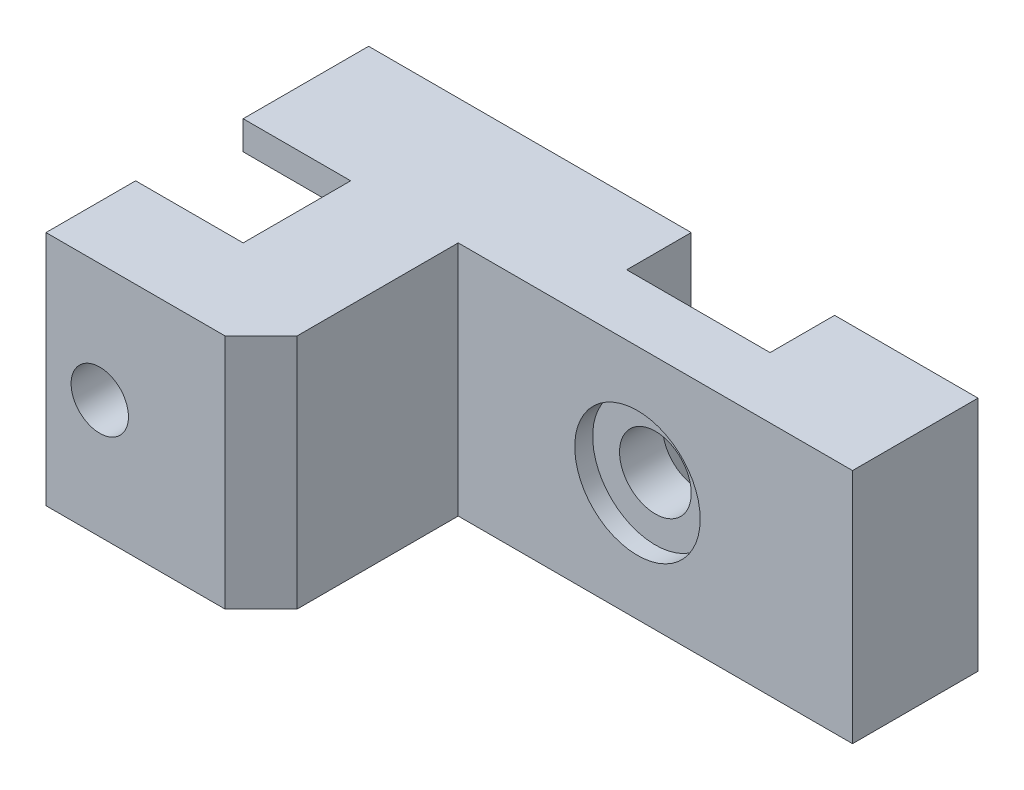
ISO-10303-21;
HEADER;
FILE_DESCRIPTION(('STEP AP214'),'2;1');
FILE_NAME('part.step','',(''),(''),'','','');
FILE_SCHEMA(('AUTOMOTIVE_DESIGN { 1 0 10303 214 1 1 1 1 }'));
ENDSEC;
DATA;
#1=APPLICATION_CONTEXT('core data for automotive mechanical design processes');
#2=APPLICATION_PROTOCOL_DEFINITION('international standard','automotive_design',2000,#1);
#3=PRODUCT_CONTEXT('',#1,'mechanical');
#4=PRODUCT('Part','Part','',(#3));
#5=PRODUCT_RELATED_PRODUCT_CATEGORY('part','',(#4));
#6=PRODUCT_DEFINITION_FORMATION('','',#4);
#7=PRODUCT_DEFINITION_CONTEXT('part definition',#1,'design');
#8=PRODUCT_DEFINITION('design','',#6,#7);
#9=PRODUCT_DEFINITION_SHAPE('','',#8);
#10=(LENGTH_UNIT() NAMED_UNIT(*) SI_UNIT(.MILLI.,.METRE.));
#11=(NAMED_UNIT(*) PLANE_ANGLE_UNIT() SI_UNIT($,.RADIAN.));
#12=(NAMED_UNIT(*) SI_UNIT($,.STERADIAN.) SOLID_ANGLE_UNIT());
#13=UNCERTAINTY_MEASURE_WITH_UNIT(LENGTH_MEASURE(1.E-05),#10,'distance_accuracy_value','');
#14=(GEOMETRIC_REPRESENTATION_CONTEXT(3) GLOBAL_UNCERTAINTY_ASSIGNED_CONTEXT((#13)) GLOBAL_UNIT_ASSIGNED_CONTEXT((#10,
#11,#12)) REPRESENTATION_CONTEXT('',''));
#15=CARTESIAN_POINT('',(0.,0.,0.));
#16=DIRECTION('',(0.,0.,1.));
#17=DIRECTION('',(1.,0.,0.));
#18=AXIS2_PLACEMENT_3D('',#15,#16,#17);
#19=CARTESIAN_POINT('',(0.,0.,35.));
#20=DIRECTION('',(0.,0.,1.));
#21=DIRECTION('',(1.,0.,0.));
#22=AXIS2_PLACEMENT_3D('',#19,#20,#21);
#23=PLANE('',#22);
#24=CARTESIAN_POINT('',(110.,33.,35.));
#25=DIRECTION('',(0.,0.,1.));
#26=DIRECTION('',(1.,0.,0.));
#27=AXIS2_PLACEMENT_3D('',#24,#25,#26);
#28=CIRCLE('',#27,17.5);
#29=CARTESIAN_POINT('',(127.5,33.,35.));
#30=VERTEX_POINT('',#29);
#31=EDGE_CURVE('E251',#30,#30,#28,.T.);
#32=ORIENTED_EDGE('',*,*,#31,.F.);
#33=EDGE_LOOP('',(#32));
#34=FACE_BOUND('',#33,.T.);
#35=DIRECTION('',(-1.,0.,0.));
#36=VECTOR('',#35,1.);
#37=CARTESIAN_POINT('',(170.,66.,35.));
#38=LINE('',#37,#36);
#39=CARTESIAN_POINT('',(170.,66.,35.));
#40=VERTEX_POINT('',#39);
#41=CARTESIAN_POINT('',(60.,66.,35.));
#42=VERTEX_POINT('',#41);
#43=EDGE_CURVE('E291',#40,#42,#38,.T.);
#44=ORIENTED_EDGE('',*,*,#43,.T.);
#45=DIRECTION('',(0.,-1.,0.));
#46=VECTOR('',#45,1.);
#47=CARTESIAN_POINT('',(60.,66.,35.));
#48=LINE('',#47,#46);
#49=CARTESIAN_POINT('',(60.,0.,35.));
#50=VERTEX_POINT('',#49);
#51=EDGE_CURVE('E230',#42,#50,#48,.T.);
#52=ORIENTED_EDGE('',*,*,#51,.T.);
#53=DIRECTION('',(1.,0.,0.));
#54=VECTOR('',#53,1.);
#55=CARTESIAN_POINT('',(0.,0.,35.));
#56=LINE('',#55,#54);
#57=CARTESIAN_POINT('',(170.,0.,35.));
#58=VERTEX_POINT('',#57);
#59=EDGE_CURVE('E288',#50,#58,#56,.T.);
#60=ORIENTED_EDGE('',*,*,#59,.T.);
#61=DIRECTION('',(0.,1.,0.));
#62=VECTOR('',#61,1.);
#63=CARTESIAN_POINT('',(170.,0.,35.));
#64=LINE('',#63,#62);
#65=EDGE_CURVE('E293',#58,#40,#64,.T.);
#66=ORIENTED_EDGE('',*,*,#65,.T.);
#67=EDGE_LOOP('',(#44,#52,#60,#66));
#68=FACE_BOUND('',#67,.T.);
#69=ADVANCED_FACE('F50',(#34,#68),#23,.T.);
#70=CARTESIAN_POINT('',(0.,0.,35.));
#71=VERTEX_POINT('',#70);
#72=CARTESIAN_POINT('',(30.,0.,35.));
#73=VERTEX_POINT('',#72);
#74=EDGE_CURVE('E289',#71,#73,#56,.T.);
#75=ORIENTED_EDGE('',*,*,#74,.T.);
#76=DIRECTION('',(0.,-1.,0.));
#77=VECTOR('',#76,1.);
#78=CARTESIAN_POINT('',(30.,66.,35.));
#79=LINE('',#78,#77);
#80=CARTESIAN_POINT('',(30.,7.99999999999999,35.));
#81=VERTEX_POINT('',#80);
#82=EDGE_CURVE('E234',#81,#73,#79,.T.);
#83=ORIENTED_EDGE('',*,*,#82,.F.);
#84=DIRECTION('',(-1.,0.,0.));
#85=VECTOR('',#84,1.);
#86=CARTESIAN_POINT('',(30.,7.99999999999999,35.));
#87=LINE('',#86,#85);
#88=CARTESIAN_POINT('',(0.,7.99999999999999,35.));
#89=VERTEX_POINT('',#88);
#90=EDGE_CURVE('E244',#81,#89,#87,.T.);
#91=ORIENTED_EDGE('',*,*,#90,.T.);
#92=DIRECTION('',(0.,-1.,0.));
#93=VECTOR('',#92,1.);
#94=CARTESIAN_POINT('',(0.,66.,35.));
#95=LINE('',#94,#93);
#96=EDGE_CURVE('E103',#89,#71,#95,.T.);
#97=ORIENTED_EDGE('',*,*,#96,.T.);
#98=EDGE_LOOP('',(#75,#83,#91,#97));
#99=FACE_BOUND('',#98,.T.);
#100=ADVANCED_FACE('F343',(#99),#23,.T.);
#101=DIRECTION('',(-1.,0.,0.));
#102=VECTOR('',#101,1.);
#103=CARTESIAN_POINT('',(30.,58.,35.));
#104=LINE('',#103,#102);
#105=CARTESIAN_POINT('',(30.,58.,35.));
#106=VERTEX_POINT('',#105);
#107=CARTESIAN_POINT('',(0.,58.,35.));
#108=VERTEX_POINT('',#107);
#109=EDGE_CURVE('E250',#106,#108,#104,.T.);
#110=ORIENTED_EDGE('',*,*,#109,.F.);
#111=CARTESIAN_POINT('',(30.,66.,35.));
#112=VERTEX_POINT('',#111);
#113=EDGE_CURVE('E235',#112,#106,#79,.T.);
#114=ORIENTED_EDGE('',*,*,#113,.F.);
#115=CARTESIAN_POINT('',(0.,66.,35.));
#116=VERTEX_POINT('',#115);
#117=EDGE_CURVE('E72',#112,#116,#38,.T.);
#118=ORIENTED_EDGE('',*,*,#117,.T.);
#119=EDGE_CURVE('E287',#116,#108,#95,.T.);
#120=ORIENTED_EDGE('',*,*,#119,.T.);
#121=EDGE_LOOP('',(#110,#114,#118,#120));
#122=FACE_BOUND('',#121,.T.);
#123=ADVANCED_FACE('F349',(#122),#23,.T.);
#124=CARTESIAN_POINT('',(0.,0.,0.));
#125=DIRECTION('',(0.,0.,1.));
#126=DIRECTION('',(1.,0.,0.));
#127=AXIS2_PLACEMENT_3D('',#124,#125,#126);
#128=PLANE('',#127);
#129=DIRECTION('',(1.,0.,0.));
#130=VECTOR('',#129,1.);
#131=CARTESIAN_POINT('',(0.,0.,0.));
#132=LINE('',#131,#130);
#133=CARTESIAN_POINT('',(130.,0.,0.));
#134=VERTEX_POINT('',#133);
#135=CARTESIAN_POINT('',(170.,0.,0.));
#136=VERTEX_POINT('',#135);
#137=EDGE_CURVE('E299',#134,#136,#132,.T.);
#138=ORIENTED_EDGE('',*,*,#137,.F.);
#139=DIRECTION('',(0.,-1.,0.));
#140=VECTOR('',#139,1.);
#141=CARTESIAN_POINT('',(130.,66.,0.));
#142=LINE('',#141,#140);
#143=CARTESIAN_POINT('',(130.,66.,0.));
#144=VERTEX_POINT('',#143);
#145=EDGE_CURVE('E281',#144,#134,#142,.T.);
#146=ORIENTED_EDGE('',*,*,#145,.F.);
#147=DIRECTION('',(-1.,0.,0.));
#148=VECTOR('',#147,1.);
#149=CARTESIAN_POINT('',(170.,66.,0.));
#150=LINE('',#149,#148);
#151=CARTESIAN_POINT('',(170.,66.,0.));
#152=VERTEX_POINT('',#151);
#153=EDGE_CURVE('E304',#152,#144,#150,.T.);
#154=ORIENTED_EDGE('',*,*,#153,.F.);
#155=DIRECTION('',(0.,1.,0.));
#156=VECTOR('',#155,1.);
#157=CARTESIAN_POINT('',(170.,0.,0.));
#158=LINE('',#157,#156);
#159=EDGE_CURVE('E303',#136,#152,#158,.T.);
#160=ORIENTED_EDGE('',*,*,#159,.F.);
#161=EDGE_LOOP('',(#138,#146,#154,#160));
#162=FACE_BOUND('',#161,.T.);
#163=ADVANCED_FACE('F325',(#162),#128,.F.);
#164=CARTESIAN_POINT('',(0.,66.,35.));
#165=DIRECTION('',(1.,0.,0.));
#166=DIRECTION('',(0.,0.,-1.));
#167=AXIS2_PLACEMENT_3D('',#164,#165,#166);
#168=PLANE('',#167);
#169=ORIENTED_EDGE('',*,*,#96,.F.);
#170=CARTESIAN_POINT('',(0.,33.,35.));
#171=DIRECTION('',(-1.,0.,0.));
#172=DIRECTION('',(0.,0.,1.));
#173=AXIS2_PLACEMENT_3D('',#170,#171,#172);
#174=CIRCLE('',#173,25.);
#175=EDGE_CURVE('E226',#108,#89,#174,.T.);
#176=ORIENTED_EDGE('',*,*,#175,.F.);
#177=ORIENTED_EDGE('',*,*,#119,.F.);
#178=DIRECTION('',(0.,0.,-1.));
#179=VECTOR('',#178,1.);
#180=CARTESIAN_POINT('',(0.,66.,35.));
#181=LINE('',#180,#179);
#182=CARTESIAN_POINT('',(0.,66.,0.));
#183=VERTEX_POINT('',#182);
#184=EDGE_CURVE('E298',#116,#183,#181,.T.);
#185=ORIENTED_EDGE('',*,*,#184,.T.);
#186=DIRECTION('',(0.,-1.,0.));
#187=VECTOR('',#186,1.);
#188=CARTESIAN_POINT('',(0.,66.,0.));
#189=LINE('',#188,#187);
#190=CARTESIAN_POINT('',(0.,0.,0.));
#191=VERTEX_POINT('',#190);
#192=EDGE_CURVE('E278',#183,#191,#189,.T.);
#193=ORIENTED_EDGE('',*,*,#192,.T.);
#194=DIRECTION('',(0.,0.,-1.));
#195=VECTOR('',#194,1.);
#196=CARTESIAN_POINT('',(0.,0.,35.));
#197=LINE('',#196,#195);
#198=EDGE_CURVE('E11',#71,#191,#197,.T.);
#199=ORIENTED_EDGE('',*,*,#198,.F.);
#200=EDGE_LOOP('',(#169,#176,#177,#185,#193,#199));
#201=FACE_BOUND('',#200,.T.);
#202=ADVANCED_FACE('F47',(#201),#168,.F.);
#203=CARTESIAN_POINT('',(0.,0.,35.));
#204=DIRECTION('',(0.,1.,0.));
#205=DIRECTION('',(0.,0.,1.));
#206=AXIS2_PLACEMENT_3D('',#203,#204,#205);
#207=PLANE('',#206);
#208=DIRECTION('',(-1.,0.,0.));
#209=VECTOR('',#208,1.);
#210=CARTESIAN_POINT('',(0.,0.,18.));
#211=LINE('',#210,#209);
#212=CARTESIAN_POINT('',(130.,0.,18.));
#213=VERTEX_POINT('',#212);
#214=CARTESIAN_POINT('',(90.,0.,18.));
#215=VERTEX_POINT('',#214);
#216=EDGE_CURVE('E258',#213,#215,#211,.T.);
#217=ORIENTED_EDGE('',*,*,#216,.F.);
#218=DIRECTION('',(0.,0.,1.));
#219=VECTOR('',#218,1.);
#220=CARTESIAN_POINT('',(130.,0.,0.));
#221=LINE('',#220,#219);
#222=EDGE_CURVE('E270',#134,#213,#221,.T.);
#223=ORIENTED_EDGE('',*,*,#222,.F.);
#224=ORIENTED_EDGE('',*,*,#137,.T.);
#225=DIRECTION('',(0.,0.,-1.));
#226=VECTOR('',#225,1.);
#227=CARTESIAN_POINT('',(170.,0.,35.));
#228=LINE('',#227,#226);
#229=EDGE_CURVE('E54',#58,#136,#228,.T.);
#230=ORIENTED_EDGE('',*,*,#229,.F.);
#231=ORIENTED_EDGE('',*,*,#59,.F.);
#232=DIRECTION('',(0.,0.,-1.));
#233=VECTOR('',#232,1.);
#234=CARTESIAN_POINT('',(60.,0.,0.));
#235=LINE('',#234,#233);
#236=CARTESIAN_POINT('',(60.,0.,80.));
#237=VERTEX_POINT('',#236);
#238=EDGE_CURVE('E201',#237,#50,#235,.T.);
#239=ORIENTED_EDGE('',*,*,#238,.F.);
#240=DIRECTION('',(0.707106781186548,0.,-0.707106781186547));
#241=VECTOR('',#240,1.);
#242=CARTESIAN_POINT('',(70.,0.,70.));
#243=LINE('',#242,#241);
#244=CARTESIAN_POINT('',(50.,0.,90.));
#245=VERTEX_POINT('',#244);
#246=EDGE_CURVE('E218',#245,#237,#243,.T.);
#247=ORIENTED_EDGE('',*,*,#246,.F.);
#248=DIRECTION('',(1.,0.,0.));
#249=VECTOR('',#248,1.);
#250=CARTESIAN_POINT('',(0.,0.,90.));
#251=LINE('',#250,#249);
#252=CARTESIAN_POINT('',(0.,0.,90.));
#253=VERTEX_POINT('',#252);
#254=EDGE_CURVE('E193',#253,#245,#251,.T.);
#255=ORIENTED_EDGE('',*,*,#254,.F.);
#256=DIRECTION('',(0.,0.,1.));
#257=VECTOR('',#256,1.);
#258=CARTESIAN_POINT('',(0.,0.,0.));
#259=LINE('',#258,#257);
#260=CARTESIAN_POINT('',(0.,0.,65.));
#261=VERTEX_POINT('',#260);
#262=EDGE_CURVE('E225',#261,#253,#259,.T.);
#263=ORIENTED_EDGE('',*,*,#262,.F.);
#264=DIRECTION('',(-1.,0.,0.));
#265=VECTOR('',#264,1.);
#266=CARTESIAN_POINT('',(0.,0.,65.));
#267=LINE('',#266,#265);
#268=CARTESIAN_POINT('',(30.,0.,65.));
#269=VERTEX_POINT('',#268);
#270=EDGE_CURVE('E224',#269,#261,#267,.T.);
#271=ORIENTED_EDGE('',*,*,#270,.F.);
#272=DIRECTION('',(0.,0.,1.));
#273=VECTOR('',#272,1.);
#274=CARTESIAN_POINT('',(30.,0.,0.));
#275=LINE('',#274,#273);
#276=EDGE_CURVE('E210',#73,#269,#275,.T.);
#277=ORIENTED_EDGE('',*,*,#276,.F.);
#278=ORIENTED_EDGE('',*,*,#74,.F.);
#279=ORIENTED_EDGE('',*,*,#198,.T.);
#280=CARTESIAN_POINT('',(90.,0.,0.));
#281=VERTEX_POINT('',#280);
#282=EDGE_CURVE('E297',#191,#281,#132,.T.);
#283=ORIENTED_EDGE('',*,*,#282,.T.);
#284=DIRECTION('',(0.,0.,-1.));
#285=VECTOR('',#284,1.);
#286=CARTESIAN_POINT('',(90.,0.,0.));
#287=LINE('',#286,#285);
#288=EDGE_CURVE('E65',#215,#281,#287,.T.);
#289=ORIENTED_EDGE('',*,*,#288,.F.);
#290=EDGE_LOOP('',(#217,#223,#224,#230,#231,#239,#247,#255,#263,#271,#277,#278,#279,#283,#289));
#291=FACE_BOUND('',#290,.T.);
#292=ADVANCED_FACE('F329',(#291),#207,.F.);
#293=CARTESIAN_POINT('',(170.,0.,35.));
#294=DIRECTION('',(-1.,0.,0.));
#295=DIRECTION('',(0.,0.,1.));
#296=AXIS2_PLACEMENT_3D('',#293,#294,#295);
#297=PLANE('',#296);
#298=ORIENTED_EDGE('',*,*,#159,.T.);
#299=DIRECTION('',(0.,0.,-1.));
#300=VECTOR('',#299,1.);
#301=CARTESIAN_POINT('',(170.,66.,35.));
#302=LINE('',#301,#300);
#303=EDGE_CURVE('E308',#40,#152,#302,.T.);
#304=ORIENTED_EDGE('',*,*,#303,.F.);
#305=ORIENTED_EDGE('',*,*,#65,.F.);
#306=ORIENTED_EDGE('',*,*,#229,.T.);
#307=EDGE_LOOP('',(#298,#304,#305,#306));
#308=FACE_BOUND('',#307,.T.);
#309=ADVANCED_FACE('F314',(#308),#297,.F.);
#310=CARTESIAN_POINT('',(170.,66.,35.));
#311=DIRECTION('',(0.,-1.,0.));
#312=DIRECTION('',(0.,0.,-1.));
#313=AXIS2_PLACEMENT_3D('',#310,#311,#312);
#314=PLANE('',#313);
#315=ORIENTED_EDGE('',*,*,#153,.T.);
#316=DIRECTION('',(0.,0.,1.));
#317=VECTOR('',#316,1.);
#318=CARTESIAN_POINT('',(130.,66.,0.));
#319=LINE('',#318,#317);
#320=CARTESIAN_POINT('',(130.,66.,18.));
#321=VERTEX_POINT('',#320);
#322=EDGE_CURVE('E269',#144,#321,#319,.T.);
#323=ORIENTED_EDGE('',*,*,#322,.T.);
#324=DIRECTION('',(-1.,0.,0.));
#325=VECTOR('',#324,1.);
#326=CARTESIAN_POINT('',(0.,66.,18.));
#327=LINE('',#326,#325);
#328=CARTESIAN_POINT('',(90.,66.,18.));
#329=VERTEX_POINT('',#328);
#330=EDGE_CURVE('E264',#321,#329,#327,.T.);
#331=ORIENTED_EDGE('',*,*,#330,.T.);
#332=DIRECTION('',(0.,0.,-1.));
#333=VECTOR('',#332,1.);
#334=CARTESIAN_POINT('',(90.,66.,0.));
#335=LINE('',#334,#333);
#336=CARTESIAN_POINT('',(90.,66.,0.));
#337=VERTEX_POINT('',#336);
#338=EDGE_CURVE('E267',#329,#337,#335,.T.);
#339=ORIENTED_EDGE('',*,*,#338,.T.);
#340=EDGE_CURVE('E93',#337,#183,#150,.T.);
#341=ORIENTED_EDGE('',*,*,#340,.T.);
#342=ORIENTED_EDGE('',*,*,#184,.F.);
#343=ORIENTED_EDGE('',*,*,#117,.F.);
#344=DIRECTION('',(0.,0.,1.));
#345=VECTOR('',#344,1.);
#346=CARTESIAN_POINT('',(30.,66.,0.));
#347=LINE('',#346,#345);
#348=CARTESIAN_POINT('',(30.,66.,65.));
#349=VERTEX_POINT('',#348);
#350=EDGE_CURVE('E216',#112,#349,#347,.T.);
#351=ORIENTED_EDGE('',*,*,#350,.T.);
#352=DIRECTION('',(-1.,0.,0.));
#353=VECTOR('',#352,1.);
#354=CARTESIAN_POINT('',(0.,66.,65.));
#355=LINE('',#354,#353);
#356=CARTESIAN_POINT('',(0.,66.,65.));
#357=VERTEX_POINT('',#356);
#358=EDGE_CURVE('E211',#349,#357,#355,.T.);
#359=ORIENTED_EDGE('',*,*,#358,.T.);
#360=DIRECTION('',(0.,0.,1.));
#361=VECTOR('',#360,1.);
#362=CARTESIAN_POINT('',(0.,66.,0.));
#363=LINE('',#362,#361);
#364=CARTESIAN_POINT('',(0.,66.,90.));
#365=VERTEX_POINT('',#364);
#366=EDGE_CURVE('E187',#357,#365,#363,.T.);
#367=ORIENTED_EDGE('',*,*,#366,.T.);
#368=DIRECTION('',(1.,0.,0.));
#369=VECTOR('',#368,1.);
#370=CARTESIAN_POINT('',(0.,66.,90.));
#371=LINE('',#370,#369);
#372=CARTESIAN_POINT('',(50.,66.,90.));
#373=VERTEX_POINT('',#372);
#374=EDGE_CURVE('E178',#365,#373,#371,.T.);
#375=ORIENTED_EDGE('',*,*,#374,.T.);
#376=DIRECTION('',(0.707106781186548,0.,-0.707106781186547));
#377=VECTOR('',#376,1.);
#378=CARTESIAN_POINT('',(70.,66.,70.));
#379=LINE('',#378,#377);
#380=CARTESIAN_POINT('',(60.,66.,80.));
#381=VERTEX_POINT('',#380);
#382=EDGE_CURVE('E182',#373,#381,#379,.T.);
#383=ORIENTED_EDGE('',*,*,#382,.T.);
#384=DIRECTION('',(0.,0.,-1.));
#385=VECTOR('',#384,1.);
#386=CARTESIAN_POINT('',(60.,66.,0.));
#387=LINE('',#386,#385);
#388=EDGE_CURVE('E200',#381,#42,#387,.T.);
#389=ORIENTED_EDGE('',*,*,#388,.T.);
#390=ORIENTED_EDGE('',*,*,#43,.F.);
#391=ORIENTED_EDGE('',*,*,#303,.T.);
#392=EDGE_LOOP('',(#315,#323,#331,#339,#341,#342,#343,#351,#359,#367,#375,#383,#389,#390,#391));
#393=FACE_BOUND('',#392,.T.);
#394=ADVANCED_FACE('F181',(#393),#314,.F.);
#395=ORIENTED_EDGE('',*,*,#340,.F.);
#396=DIRECTION('',(0.,-1.,0.));
#397=VECTOR('',#396,1.);
#398=CARTESIAN_POINT('',(90.,66.,0.));
#399=LINE('',#398,#397);
#400=EDGE_CURVE('E284',#337,#281,#399,.T.);
#401=ORIENTED_EDGE('',*,*,#400,.T.);
#402=ORIENTED_EDGE('',*,*,#282,.F.);
#403=ORIENTED_EDGE('',*,*,#192,.F.);
#404=EDGE_LOOP('',(#395,#401,#402,#403));
#405=FACE_BOUND('',#404,.T.);
#406=ADVANCED_FACE('F365',(#405),#128,.F.);
#407=CARTESIAN_POINT('',(0.,66.,18.));
#408=DIRECTION('',(0.,0.,1.));
#409=DIRECTION('',(1.,0.,0.));
#410=AXIS2_PLACEMENT_3D('',#407,#408,#409);
#411=PLANE('',#410);
#412=CARTESIAN_POINT('',(110.,33.,18.));
#413=DIRECTION('',(0.,0.,1.));
#414=DIRECTION('',(1.,0.,0.));
#415=AXIS2_PLACEMENT_3D('',#412,#413,#414);
#416=CIRCLE('',#415,9.99999999999999);
#417=CARTESIAN_POINT('',(120.,33.,18.));
#418=VERTEX_POINT('',#417);
#419=EDGE_CURVE('E252',#418,#418,#416,.T.);
#420=ORIENTED_EDGE('',*,*,#419,.T.);
#421=EDGE_LOOP('',(#420));
#422=FACE_BOUND('',#421,.T.);
#423=ORIENTED_EDGE('',*,*,#216,.T.);
#424=DIRECTION('',(0.,-1.,0.));
#425=VECTOR('',#424,1.);
#426=CARTESIAN_POINT('',(90.,66.,18.));
#427=LINE('',#426,#425);
#428=EDGE_CURVE('E275',#329,#215,#427,.T.);
#429=ORIENTED_EDGE('',*,*,#428,.F.);
#430=ORIENTED_EDGE('',*,*,#330,.F.);
#431=DIRECTION('',(0.,-1.,0.));
#432=VECTOR('',#431,1.);
#433=CARTESIAN_POINT('',(130.,66.,18.));
#434=LINE('',#433,#432);
#435=EDGE_CURVE('E279',#321,#213,#434,.T.);
#436=ORIENTED_EDGE('',*,*,#435,.T.);
#437=EDGE_LOOP('',(#423,#429,#430,#436));
#438=FACE_BOUND('',#437,.T.);
#439=ADVANCED_FACE('F381',(#422,#438),#411,.F.);
#440=CARTESIAN_POINT('',(130.,66.,0.));
#441=DIRECTION('',(1.,0.,0.));
#442=DIRECTION('',(0.,0.,-1.));
#443=AXIS2_PLACEMENT_3D('',#440,#441,#442);
#444=PLANE('',#443);
#445=ORIENTED_EDGE('',*,*,#222,.T.);
#446=ORIENTED_EDGE('',*,*,#435,.F.);
#447=ORIENTED_EDGE('',*,*,#322,.F.);
#448=ORIENTED_EDGE('',*,*,#145,.T.);
#449=EDGE_LOOP('',(#445,#446,#447,#448));
#450=FACE_BOUND('',#449,.T.);
#451=ADVANCED_FACE('F390',(#450),#444,.F.);
#452=CARTESIAN_POINT('',(90.,66.,0.));
#453=DIRECTION('',(-1.,0.,0.));
#454=DIRECTION('',(0.,0.,1.));
#455=AXIS2_PLACEMENT_3D('',#452,#453,#454);
#456=PLANE('',#455);
#457=ORIENTED_EDGE('',*,*,#288,.T.);
#458=ORIENTED_EDGE('',*,*,#400,.F.);
#459=ORIENTED_EDGE('',*,*,#338,.F.);
#460=ORIENTED_EDGE('',*,*,#428,.T.);
#461=EDGE_LOOP('',(#457,#458,#459,#460));
#462=FACE_BOUND('',#461,.T.);
#463=ADVANCED_FACE('F382',(#462),#456,.F.);
#464=CARTESIAN_POINT('',(110.,33.,30.));
#465=DIRECTION('',(0.,0.,1.));
#466=DIRECTION('',(1.,0.,0.));
#467=AXIS2_PLACEMENT_3D('',#464,#465,#466);
#468=CYLINDRICAL_SURFACE('',#467,17.5);
#469=CARTESIAN_POINT('',(110.,33.,30.));
#470=DIRECTION('',(0.,0.,1.));
#471=DIRECTION('',(1.,0.,0.));
#472=AXIS2_PLACEMENT_3D('',#469,#470,#471);
#473=CIRCLE('',#472,17.5);
#474=CARTESIAN_POINT('',(127.5,33.,30.));
#475=VERTEX_POINT('',#474);
#476=EDGE_CURVE('E260',#475,#475,#473,.T.);
#477=ORIENTED_EDGE('',*,*,#476,.F.);
#478=EDGE_LOOP('',(#477));
#479=FACE_BOUND('',#478,.T.);
#480=ORIENTED_EDGE('',*,*,#31,.T.);
#481=EDGE_LOOP('',(#480));
#482=FACE_BOUND('',#481,.T.);
#483=ADVANCED_FACE('F394',(#479,#482),#468,.F.);
#484=CARTESIAN_POINT('',(110.,33.,30.));
#485=DIRECTION('',(0.,0.,1.));
#486=DIRECTION('',(1.,0.,0.));
#487=AXIS2_PLACEMENT_3D('',#484,#485,#486);
#488=PLANE('',#487);
#489=CARTESIAN_POINT('',(110.,33.,30.));
#490=DIRECTION('',(0.,0.,1.));
#491=DIRECTION('',(1.,0.,0.));
#492=AXIS2_PLACEMENT_3D('',#489,#490,#491);
#493=CIRCLE('',#492,9.99999999999999);
#494=CARTESIAN_POINT('',(120.,33.,30.));
#495=VERTEX_POINT('',#494);
#496=EDGE_CURVE('E248',#495,#495,#493,.T.);
#497=ORIENTED_EDGE('',*,*,#496,.F.);
#498=EDGE_LOOP('',(#497));
#499=FACE_BOUND('',#498,.T.);
#500=ORIENTED_EDGE('',*,*,#476,.T.);
#501=EDGE_LOOP('',(#500));
#502=FACE_BOUND('',#501,.T.);
#503=ADVANCED_FACE('F399',(#499,#502),#488,.T.);
#504=CARTESIAN_POINT('',(110.,33.,18.));
#505=DIRECTION('',(0.,0.,1.));
#506=DIRECTION('',(1.,0.,0.));
#507=AXIS2_PLACEMENT_3D('',#504,#505,#506);
#508=CYLINDRICAL_SURFACE('',#507,9.99999999999999);
#509=ORIENTED_EDGE('',*,*,#419,.F.);
#510=EDGE_LOOP('',(#509));
#511=FACE_BOUND('',#510,.T.);
#512=ORIENTED_EDGE('',*,*,#496,.T.);
#513=EDGE_LOOP('',(#512));
#514=FACE_BOUND('',#513,.T.);
#515=ADVANCED_FACE('F401',(#511,#514),#508,.F.);
#516=CARTESIAN_POINT('',(30.,33.,35.));
#517=DIRECTION('',(-1.,0.,0.));
#518=DIRECTION('',(0.,0.,1.));
#519=AXIS2_PLACEMENT_3D('',#516,#517,#518);
#520=CYLINDRICAL_SURFACE('',#519,25.);
#521=ORIENTED_EDGE('',*,*,#175,.T.);
#522=ORIENTED_EDGE('',*,*,#90,.F.);
#523=CARTESIAN_POINT('',(30.,33.,35.));
#524=DIRECTION('',(-1.,0.,0.));
#525=DIRECTION('',(0.,0.,1.));
#526=AXIS2_PLACEMENT_3D('',#523,#524,#525);
#527=CIRCLE('',#526,25.);
#528=EDGE_CURVE('E245',#106,#81,#527,.T.);
#529=ORIENTED_EDGE('',*,*,#528,.F.);
#530=ORIENTED_EDGE('',*,*,#109,.T.);
#531=EDGE_LOOP('',(#521,#522,#529,#530));
#532=FACE_BOUND('',#531,.T.);
#533=ADVANCED_FACE('F368',(#532),#520,.F.);
#534=CARTESIAN_POINT('',(30.,33.,35.));
#535=DIRECTION('',(-1.,0.,0.));
#536=DIRECTION('',(0.,0.,1.));
#537=AXIS2_PLACEMENT_3D('',#534,#535,#536);
#538=PLANE('',#537);
#539=ORIENTED_EDGE('',*,*,#528,.T.);
#540=ORIENTED_EDGE('',*,*,#82,.T.);
#541=ORIENTED_EDGE('',*,*,#276,.T.);
#542=DIRECTION('',(0.,-1.,0.));
#543=VECTOR('',#542,1.);
#544=CARTESIAN_POINT('',(30.,66.,65.));
#545=LINE('',#544,#543);
#546=EDGE_CURVE('E232',#349,#269,#545,.T.);
#547=ORIENTED_EDGE('',*,*,#546,.F.);
#548=ORIENTED_EDGE('',*,*,#350,.F.);
#549=ORIENTED_EDGE('',*,*,#113,.T.);
#550=EDGE_LOOP('',(#539,#540,#541,#547,#548,#549));
#551=FACE_BOUND('',#550,.T.);
#552=ADVANCED_FACE('F342',(#551),#538,.T.);
#553=CARTESIAN_POINT('',(70.,66.,70.));
#554=DIRECTION('',(-0.707106781186547,0.,-0.707106781186548));
#555=DIRECTION('',(-0.707106781186548,0.,0.707106781186547));
#556=AXIS2_PLACEMENT_3D('',#553,#554,#555);
#557=PLANE('',#556);
#558=ORIENTED_EDGE('',*,*,#246,.T.);
#559=DIRECTION('',(0.,-1.,0.));
#560=VECTOR('',#559,1.);
#561=CARTESIAN_POINT('',(60.,66.,80.));
#562=LINE('',#561,#560);
#563=EDGE_CURVE('E204',#381,#237,#562,.T.);
#564=ORIENTED_EDGE('',*,*,#563,.F.);
#565=ORIENTED_EDGE('',*,*,#382,.F.);
#566=DIRECTION('',(0.,-1.,0.));
#567=VECTOR('',#566,1.);
#568=CARTESIAN_POINT('',(50.,66.,90.));
#569=LINE('',#568,#567);
#570=EDGE_CURVE('E195',#373,#245,#569,.T.);
#571=ORIENTED_EDGE('',*,*,#570,.T.);
#572=EDGE_LOOP('',(#558,#564,#565,#571));
#573=FACE_BOUND('',#572,.T.);
#574=ADVANCED_FACE('F205',(#573),#557,.F.);
#575=CARTESIAN_POINT('',(60.,66.,0.));
#576=DIRECTION('',(-1.,0.,0.));
#577=DIRECTION('',(0.,0.,1.));
#578=AXIS2_PLACEMENT_3D('',#575,#576,#577);
#579=PLANE('',#578);
#580=ORIENTED_EDGE('',*,*,#238,.T.);
#581=ORIENTED_EDGE('',*,*,#51,.F.);
#582=ORIENTED_EDGE('',*,*,#388,.F.);
#583=ORIENTED_EDGE('',*,*,#563,.T.);
#584=EDGE_LOOP('',(#580,#581,#582,#583));
#585=FACE_BOUND('',#584,.T.);
#586=ADVANCED_FACE('F330',(#585),#579,.F.);
#587=CARTESIAN_POINT('',(0.,66.,65.));
#588=DIRECTION('',(0.,0.,1.));
#589=DIRECTION('',(1.,0.,0.));
#590=AXIS2_PLACEMENT_3D('',#587,#588,#589);
#591=PLANE('',#590);
#592=CARTESIAN_POINT('',(15.,33.,65.));
#593=DIRECTION('',(0.,0.,1.));
#594=DIRECTION('',(1.,0.,0.));
#595=AXIS2_PLACEMENT_3D('',#592,#593,#594);
#596=CIRCLE('',#595,8.);
#597=CARTESIAN_POINT('',(23.,33.,65.));
#598=VERTEX_POINT('',#597);
#599=EDGE_CURVE('E208',#598,#598,#596,.T.);
#600=ORIENTED_EDGE('',*,*,#599,.T.);
#601=EDGE_LOOP('',(#600));
#602=FACE_BOUND('',#601,.T.);
#603=ORIENTED_EDGE('',*,*,#270,.T.);
#604=DIRECTION('',(0.,-1.,0.));
#605=VECTOR('',#604,1.);
#606=CARTESIAN_POINT('',(0.,66.,65.));
#607=LINE('',#606,#605);
#608=EDGE_CURVE('E238',#357,#261,#607,.T.);
#609=ORIENTED_EDGE('',*,*,#608,.F.);
#610=ORIENTED_EDGE('',*,*,#358,.F.);
#611=ORIENTED_EDGE('',*,*,#546,.T.);
#612=EDGE_LOOP('',(#603,#609,#610,#611));
#613=FACE_BOUND('',#612,.T.);
#614=ADVANCED_FACE('F335',(#602,#613),#591,.F.);
#615=CARTESIAN_POINT('',(0.,66.,0.));
#616=DIRECTION('',(1.,0.,0.));
#617=DIRECTION('',(0.,0.,-1.));
#618=AXIS2_PLACEMENT_3D('',#615,#616,#617);
#619=PLANE('',#618);
#620=ORIENTED_EDGE('',*,*,#262,.T.);
#621=DIRECTION('',(0.,-1.,0.));
#622=VECTOR('',#621,1.);
#623=CARTESIAN_POINT('',(0.,66.,90.));
#624=LINE('',#623,#622);
#625=EDGE_CURVE('E198',#365,#253,#624,.T.);
#626=ORIENTED_EDGE('',*,*,#625,.F.);
#627=ORIENTED_EDGE('',*,*,#366,.F.);
#628=ORIENTED_EDGE('',*,*,#608,.T.);
#629=EDGE_LOOP('',(#620,#626,#627,#628));
#630=FACE_BOUND('',#629,.T.);
#631=ADVANCED_FACE('F336',(#630),#619,.F.);
#632=CARTESIAN_POINT('',(0.,66.,90.));
#633=DIRECTION('',(0.,0.,-1.));
#634=DIRECTION('',(-1.,0.,0.));
#635=AXIS2_PLACEMENT_3D('',#632,#633,#634);
#636=PLANE('',#635);
#637=CARTESIAN_POINT('',(15.,33.,90.));
#638=DIRECTION('',(0.,0.,1.));
#639=DIRECTION('',(1.,0.,0.));
#640=AXIS2_PLACEMENT_3D('',#637,#638,#639);
#641=CIRCLE('',#640,8.);
#642=CARTESIAN_POINT('',(23.,33.,90.));
#643=VERTEX_POINT('',#642);
#644=EDGE_CURVE('E655',#643,#643,#641,.T.);
#645=ORIENTED_EDGE('',*,*,#644,.F.);
#646=EDGE_LOOP('',(#645));
#647=FACE_BOUND('',#646,.T.);
#648=ORIENTED_EDGE('',*,*,#254,.T.);
#649=ORIENTED_EDGE('',*,*,#570,.F.);
#650=ORIENTED_EDGE('',*,*,#374,.F.);
#651=ORIENTED_EDGE('',*,*,#625,.T.);
#652=EDGE_LOOP('',(#648,#649,#650,#651));
#653=FACE_BOUND('',#652,.T.);
#654=ADVANCED_FACE('F194',(#647,#653),#636,.F.);
#655=CARTESIAN_POINT('',(15.,33.,24.));
#656=DIRECTION('',(0.,0.,1.));
#657=DIRECTION('',(1.,0.,0.));
#658=AXIS2_PLACEMENT_3D('',#655,#656,#657);
#659=CYLINDRICAL_SURFACE('',#658,8.);
#660=ORIENTED_EDGE('',*,*,#644,.T.);
#661=EDGE_LOOP('',(#660));
#662=FACE_BOUND('',#661,.T.);
#663=ORIENTED_EDGE('',*,*,#599,.F.);
#664=EDGE_LOOP('',(#663));
#665=FACE_BOUND('',#664,.T.);
#666=ADVANCED_FACE('F413',(#662,#665),#659,.F.);
#667=CLOSED_SHELL('',(#69,#100,#123,#163,#202,#292,#309,#394,#406,#439,#451,#463,#483,#503,#515,
#533,#552,#574,#586,#614,#631,#654,#666));
#668=MANIFOLD_SOLID_BREP('B2',#667);
#669=ADVANCED_BREP_SHAPE_REPRESENTATION('',(#18,#668),#14);
#670=SHAPE_DEFINITION_REPRESENTATION(#9,#669);
ENDSEC;
END-ISO-10303-21;
